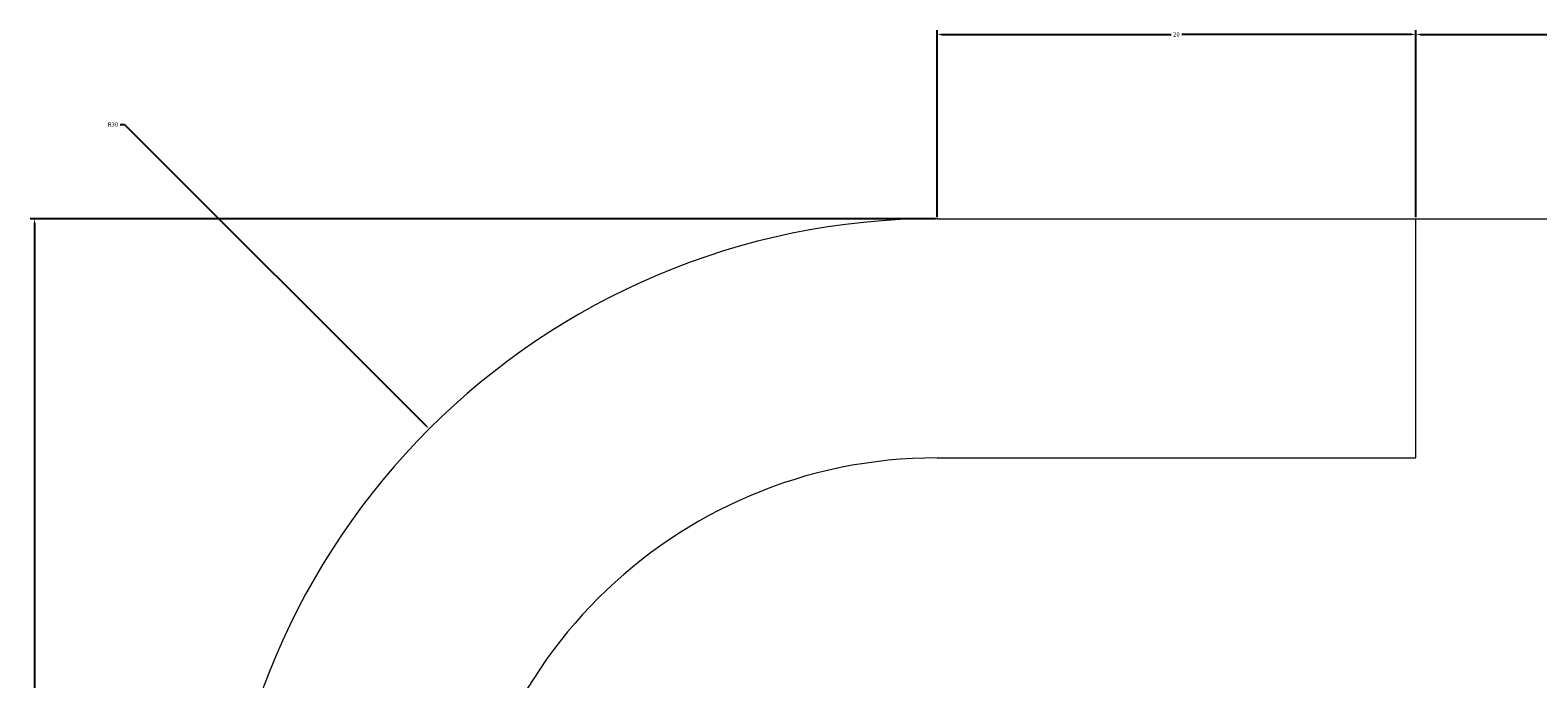
# Model space of a CAD drawing. Units: inches. Extents: x -19 to 107, y -27 to 49.
# Tile 2 of 4: x -19 to 44, y 22 to 49. Entities that reach past the tile are written whole.
import ezdxf

# ---------------------------------------------------------------- set-up
doc = ezdxf.new("R2010")
doc.units = ezdxf.units.IN
doc.header["$MEASUREMENT"] = 0
doc.layers.add('M-CONS', color=8, linetype='Continuous', lineweight=18)
doc.layers.add('M-DIMS', color=2, linetype='Continuous', lineweight=18)
doc.styles.get("Standard").update_dxf_attribs({"font": 'arial.ttf'})
doc.dimstyles.get("Standard").update_dxf_attribs({"dimtxt": 0.18, "dimasz": 0.18, "dimexe": 0.18, "dimexo": 0.0625, "dimgap": 0.09, "dimtad": 0, "dimtih": 1, "dimtoh": 1, "dimdec": 4, "dimzin": 0, "dimdsep": 46, "dimtxsty": 'Standard', "dimcen": 0.09, "dimadec": 0, "dimazin": 0, "dimtfac": 1, "dimtdec": 4, "dimtofl": 0, "dimtmove": 0, "dimatfit": 3, "dimfxl": 1, "dimtolj": 1, "dimtzin": 0, "dimarcsym": 0})

# ---------------------------------------------------------------- blocks, each defined once
blk = doc.blocks.new('*D2')
at = {"layer": 'Defpoints', "color": 0, "transparency": 16777216}
for p in [(-18.642, 40.82), (19.063, 40.82), (19.063, -19.18)]:
    blk.add_point(p, dxfattribs=at)
at = {"layer": 'M-DIMS', "color": 0, "lineweight": -2, "transparency": 16777216}
for p, q in [((19.001, 40.82), (-18.822, 40.82)), ((-18.642, 40.64), (-18.642, 11.002)), ((-18.642, -19), (-18.642, 10.638)), ((19.001, -19.18), (-18.822, -19.18))]:
    blk.add_line(p, q, dxfattribs=at)
at = {"layer": 'M-DIMS', "color": 0, "transparency": 16777216}
for points in [[(-18.672, 40.64), (-18.612, 40.64), (-18.642, 40.82)], [(-18.672, -19), (-18.612, -19), (-18.642, -19.18)]]:
    blk.add_solid(points, dxfattribs=at)
at = {"layer": 'M-DIMS', "color": 0, "transparency": 16777216, "insert": (-18.642, 10.82), "char_height": 0.18, "attachment_point": 5}
blk.add_mtext('\\A1;60', dxfattribs=at)
blk = doc.blocks.new('*D3')
at = {"layer": 'Defpoints', "color": 0, "transparency": 16777216}
for p in [(39.063, 48.525), (19.063, 40.82), (39.063, 40.82)]:
    blk.add_point(p, dxfattribs=at)
at = {"layer": 'M-DIMS', "color": 0, "lineweight": -2, "transparency": 16777216}
for p, q in [((19.063, 40.883), (19.063, 48.705)), ((19.243, 48.525), (28.843, 48.525)), ((38.883, 48.525), (29.284, 48.525)), ((39.063, 40.883), (39.063, 48.705))]:
    blk.add_line(p, q, dxfattribs=at)
at = {"layer": 'M-DIMS', "color": 0, "transparency": 16777216}
for points in [[(19.243, 48.555), (19.243, 48.495), (19.063, 48.525)], [(38.883, 48.555), (38.883, 48.495), (39.063, 48.525)]]:
    blk.add_solid(points, dxfattribs=at)
at = {"layer": 'M-DIMS', "color": 0, "transparency": 16777216, "insert": (29.063, 48.525), "char_height": 0.18, "attachment_point": 5}
blk.add_mtext('\\A1;20', dxfattribs=at)
blk = doc.blocks.new('*D4')
at = {"layer": 'Defpoints', "color": 0, "transparency": 16777216}
for p in [(84.063, 48.525), (39.063, 40.82), (84.063, 25.624)]:
    blk.add_point(p, dxfattribs=at)
at = {"layer": 'M-DIMS', "color": 0, "lineweight": -2, "transparency": 16777216}
for p, q in [((39.063, 40.883), (39.063, 48.705)), ((39.243, 48.525), (61.34, 48.525)), ((83.883, 48.525), (61.787, 48.525)), ((84.063, 25.687), (84.063, 48.705))]:
    blk.add_line(p, q, dxfattribs=at)
at = {"layer": 'M-DIMS', "color": 0, "transparency": 16777216}
for points in [[(39.243, 48.555), (39.243, 48.495), (39.063, 48.525)], [(83.883, 48.555), (83.883, 48.495), (84.063, 48.525)]]:
    blk.add_solid(points, dxfattribs=at)
at = {"layer": 'M-DIMS', "color": 0, "transparency": 16777216, "insert": (61.563, 48.525), "char_height": 0.18, "attachment_point": 5}
blk.add_mtext('\\A1;45', dxfattribs=at)
blk = doc.blocks.new('*D9')
at = {"layer": 'Defpoints', "color": 0, "transparency": 16777216}
for p in [(-2.151, 32.031), (19.063, 10.82)]:
    blk.add_point(p, dxfattribs=at)
at = {"layer": 'M-DIMS', "color": 0, "lineweight": -2, "transparency": 16777216}
for p, q in [((-15.06, 44.758), (-14.88, 44.758)), ((-14.88, 44.758), (-2.279, 32.159)), ((18.973, 10.82), (19.153, 10.82)), ((19.063, 10.73), (19.063, 10.91))]:
    blk.add_line(p, q, dxfattribs=at)
at = {"layer": 'M-DIMS', "color": 0, "transparency": 16777216}
blk.add_solid([(-2.258, 32.18), (-2.3, 32.138), (-2.151, 32.031)], dxfattribs=at)
at = {"layer": 'M-DIMS', "color": 0, "transparency": 16777216, "insert": (-15.365, 44.758), "char_height": 0.18, "attachment_point": 5}
blk.add_mtext('\\A1;R30', dxfattribs=at)

msp = doc.modelspace()

# ---------------------------------------------------------------- linework, layer by layer
at = {"layer": 'M-CONS'}
for p, q in [((19.0635, 40.82), (99.0635, 40.82)), ((39.0635, 30.82, 20), (39.0635, 40.82, 20)), ((19.0635, 30.82, 20), (39.0635, 30.82, 20))]:
    msp.add_line(p, q, dxfattribs=at)
for centre, radius in [((19.0635, 10.82), 30), ((19.0635, 10.82, 20), 20)]:
    msp.add_arc(centre, radius, 90, 270, dxfattribs=at)

# ---------------------------------------------------------------- dimensions: what is measured, and where the dimension line sits
at = {"layer": 'M-DIMS'}
for base, p1, p2, picture, middle in [((39.0635, 48.525), (19.0635, 40.82), (39.0635, 40.82), '*D3', (29.0635, 48.525)), ((84.0635, 48.525), (39.0635, 40.82), (84.0635, 25.6245), '*D4', (61.5635, 48.525))]:
    dim = msp.add_linear_dim(base=base, p1=p1, p2=p2, dimstyle='Standard', override={"dimdec": 0, "dimlfac": 1, "dimrnd": 0, "dimzin": 0, "dimdsep": 46, "dimlunit": 2}, dxfattribs=at)
    dim.commit()
    dim.dimension.update_dxf_attribs({"geometry": picture, "text_midpoint": middle})
dim = msp.add_radius_dim(center=(19.0635, 10.82), mpoint=(-2.1515, 32.0315), dimstyle='Standard', override={"dimdec": 0, "dimlfac": 1, "dimrnd": 0, "dimzin": 0, "dimdsep": 46, "dimlunit": 2}, dxfattribs=at)
dim.commit()
dim.dimension.update_dxf_attribs({"geometry": '*D9', "text_midpoint": (-15.3652, 44.7583), "dimtype": 164})
dim = msp.add_linear_dim(base=(-18.6415, 40.82), p1=(19.0635, -19.18), p2=(19.0635, 40.82), angle=90, dimstyle='Standard', override={"dimdec": 0, "dimlfac": 1, "dimrnd": 0, "dimzin": 0, "dimdsep": 46, "dimlunit": 2}, dxfattribs=at)
dim.commit()
dim.dimension.update_dxf_attribs({"geometry": '*D2', "text_midpoint": (-18.6415, 10.82)})

doc.saveas('drawing.dxf')
